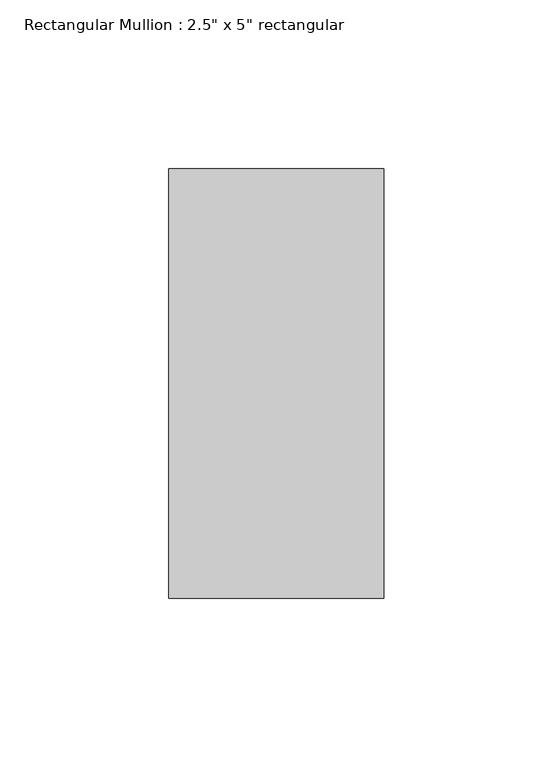
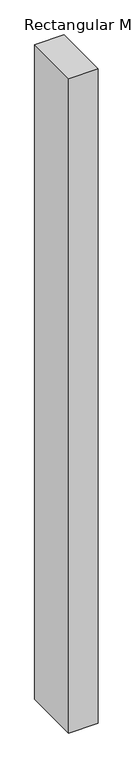
"""IFC4 building model written with IfcOpenShell, lengths in millimetres: member geometry."""

from ifc_helpers import new_model, si_unit, frame, origin, place, context, project, spatial, polyline, outline, extrude, source, transform, mapped, element, save


def member_28306602(model_context):
    return source(origin(), model_context, "Body", "SweptSolid", [
        extrude(outline(polyline([(0.0, 63.5), (0.0, -63.5), (-63.5, -63.5), (-63.5, 63.5), (0.0, 63.5)])), frame((0.0, 0.0, -1490.0142793), z_axis=(0.0, 0.0, 1.0), x_axis=(1.0, 0.0, 0.0)), (0.0, 0.0, 1.0), 1490.0142793),
    ])


if __name__ == "__main__":
    model = new_model("IFC4")
    model_context = context("Model", 3, world=origin())
    ifc_project = project(units=[si_unit("LENGTHUNIT", "METRE", prefix="MILLI")], contexts=[model_context])
    site = spatial("IfcSite", under=ifc_project)
    building = spatial("IfcBuilding", under=site)
    placement = place(None, origin())
    member_shape = member_28306602(model_context)
    element("IfcMember", 1, ObjectType="Rectangular Mullion : 2.5\" x 5\" rectangular", at=placement, inside=building, context=model_context, shape_type="MappedRepresentation", body=[
        mapped(member_shape, transform((0.0, 0.0, 0.0), x_axis=(1.0, 0.0, 0.0), y_axis=(0.0, 1.0, 0.0), z_axis=(0.0, 0.0, 1.0))),
    ])
    save(model, "model.ifc")

# Revit data of these elements
# Type "Rectangular Mullion : 2.5\" x 5\" rectangular"
#   built-in parameter 1007304 = 0.416667 (stored number, unit not read)
#   built-in parameter 1007301 = 0.104167 (stored number, unit not read)
#   built-in parameter 1007300 = 0.104167 (stored number, unit not read)
